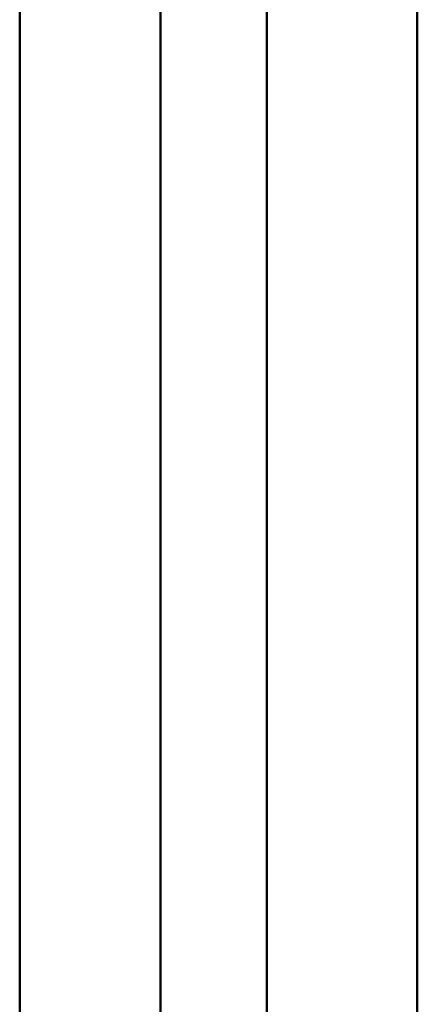
# Model space of a CAD drawing. Units: inches. Extents: x 64 to 1167, y 117 to 939.
# Tile 24 of 56: x 373.107 to 377.107, y 827.498 to 837.398. Entities that reach past the tile are written whole.
import ezdxf

# ---------------------------------------------------------------- set-up
doc = ezdxf.new("R2010")
doc.units = ezdxf.units.IN
doc.header["$MEASUREMENT"] = 0
doc.layers.add('A-WALL', color=7, linetype='Continuous', lineweight=50)

msp = doc.modelspace()

# ---------------------------------------------------------------- linework, layer by layer
at = {"layer": 'A-WALL'}
for p, q in [((377.1073, 857.1998), (377.1073, 823.3109)), ((373.1073, 847.3109), (373.1073, 785.1998)), ((374.5241, 847.3109), (374.5241, 823.3109)), ((375.595, 847.3109), (375.595, 823.3109)), ((377.1073, 847.3109), (377.1073, 785.1998))]:
    msp.add_line(p, q, dxfattribs=at)

doc.saveas('drawing.dxf')
